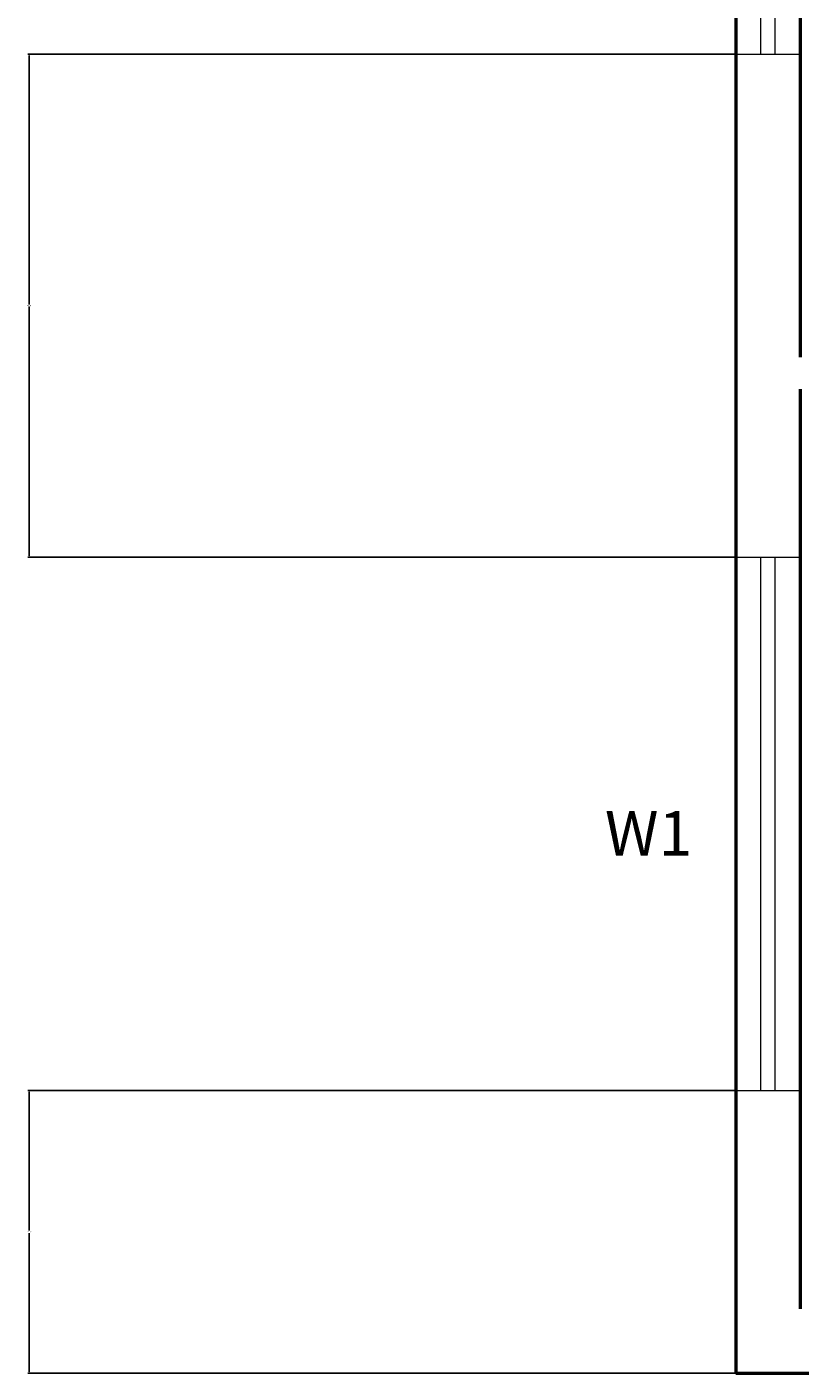
# Model space of a CAD drawing. Units: inches. Extents: x 7359 to 7979, y 33027 to 34263.
# Tile 2 of 32: x 7369 to 7478, y 33159 to 33347. Entities that reach past the tile are written whole.
import ezdxf

# ---------------------------------------------------------------- set-up
doc = ezdxf.new("R2010")
doc.units = ezdxf.units.IN
for name, color, linetype, lineweight in [('A-ANNO-DIMS', 2, 'Continuous', 18), ('A-ANNO-TEXT', 3, 'Continuous', 18), ('A-GLAZ', 4, 'Continuous', 18), ('A-WALL', 7, 'Continuous', 50)]:
    doc.layers.add(name, color=color, linetype=linetype, lineweight=lineweight)
doc.styles.get("Standard").update_dxf_attribs({"font": 'arial.ttf'})
doc.dimstyles.get("Standard").update_dxf_attribs({"dimtxt": 0.18, "dimasz": 0.18, "dimexe": 0.18, "dimexo": 0.0625, "dimgap": 0.09, "dimtad": 0, "dimtih": 1, "dimtoh": 1, "dimdec": 4, "dimzin": 0, "dimdsep": 46, "dimtxsty": 'Standard', "dimcen": 0.09, "dimadec": 0, "dimazin": 0, "dimtfac": 1, "dimtdec": 4, "dimtofl": 0, "dimtmove": 0, "dimatfit": 3, "dimfxl": 1, "dimtolj": 1, "dimtzin": 0, "dimarcsym": 0})

# ---------------------------------------------------------------- blocks, each defined once
blk = doc.blocks.new('WINDOW-W1-LIVING')
for p, q in [((0, 91.75), (9, 91.75)), ((3.5, 0), (3.5, 91.75)), ((5.5, 0), (5.5, 91.75)), ((0, 0), (9, 0))]:
    blk.add_line(p, q)
blk = doc.blocks.new('WINDOW-W1-DRAWING-SIDE')
for p, q in [((0, 74.75), (9, 74.75)), ((3.5, 0), (3.5, 74.75)), ((5.5, 0), (5.5, 74.75)), ((0, 0), (9, 0))]:
    blk.add_line(p, q)
blk = doc.blocks.new('*D79')
at = {"layer": 'A-ANNO-DIMS', "color": 0, "lineweight": -2, "transparency": 16777216}
for p, q in [((7468.66, 33198.25), (7369.54, 33198.25)), ((7369.72, 33198.07), (7369.72, 33178.64)), ((7369.72, 33158.84), (7369.72, 33178.28)), ((7468.66, 33158.66), (7369.54, 33158.66))]:
    blk.add_line(p, q, dxfattribs=at)
at = {"layer": 'A-ANNO-DIMS', "color": 0, "transparency": 16777216}
for points in [[(7369.69, 33198.07), (7369.75, 33198.07), (7369.72, 33198.25)], [(7369.69, 33158.84), (7369.75, 33158.84), (7369.72, 33158.66)]]:
    blk.add_solid(points, dxfattribs=at)
at = {"layer": 'Defpoints', "color": 0, "transparency": 16777216}
for p in [(7369.72, 33198.25), (7468.73, 33198.25), (7468.73, 33158.66)]:
    blk.add_point(p, dxfattribs=at)
at = {"layer": 'A-ANNO-DIMS', "color": 0, "transparency": 16777216, "insert": (7369.72, 33178.46), "char_height": 0.18, "attachment_point": 5}
blk.add_mtext('\\A1;39.59', dxfattribs=at)
blk = doc.blocks.new('*D80')
at = {"layer": 'A-ANNO-DIMS', "color": 0, "lineweight": -2, "transparency": 16777216}
for p, q in [((7468.66, 33343.52), (7369.54, 33343.52)), ((7369.72, 33343.34), (7369.72, 33308.44)), ((7369.72, 33273.18), (7369.72, 33308.08)), ((7468.66, 33273), (7369.54, 33273))]:
    blk.add_line(p, q, dxfattribs=at)
at = {"layer": 'A-ANNO-DIMS', "color": 0, "transparency": 16777216}
for points in [[(7369.69, 33343.34), (7369.75, 33343.34), (7369.72, 33343.52)], [(7369.69, 33273.18), (7369.75, 33273.18), (7369.72, 33273)]]:
    blk.add_solid(points, dxfattribs=at)
at = {"layer": 'Defpoints', "color": 0, "transparency": 16777216}
for p in [(7369.72, 33343.52), (7468.73, 33343.52), (7468.73, 33273)]:
    blk.add_point(p, dxfattribs=at)
at = {"layer": 'A-ANNO-DIMS', "color": 0, "transparency": 16777216, "insert": (7369.72, 33308.26), "char_height": 0.18, "attachment_point": 5}
blk.add_mtext('\\A1;70.51', dxfattribs=at)

msp = doc.modelspace()

# ---------------------------------------------------------------- linework, layer by layer
at = {"layer": 'A-WALL'}
for p, q in [((7468.7266, 33627.1623), (7468.7266, 33158.6623)), ((7477.7266, 33471.1623), (7477.7266, 33301.0623)), ((7477.7266, 33296.5623), (7477.7266, 33167.6623)), ((7468.7266, 33158.6623), (7894.1266, 33158.6623))]:
    msp.add_line(p, q, dxfattribs=at)

# ---------------------------------------------------------------- block references
at = {"layer": 'A-GLAZ'}
for name, p in [('WINDOW-W1-LIVING', (7468.7261, 33343.5154)), ('WINDOW-W1-DRAWING-SIDE', (7468.7261, 33198.2534))]:
    msp.add_blockref(name, p, dxfattribs=at)

# ---------------------------------------------------------------- texts
at = {"layer": 'A-ANNO-TEXT'}
msp.add_text('W1', height=6.25941, dxfattribs=at).set_placement((7450.3922, 33231.1644))

# ---------------------------------------------------------------- dimensions: what is measured, and where the dimension line sits
at = {"layer": 'A-ANNO-DIMS'}
for base, p1, p2, picture, middle in [((7369.7217, 33343.5157), (7468.7266, 33273.0048), (7468.7266, 33343.5157), '*D80', (7369.7217, 33308.2602)), ((7369.7217, 33198.2537), (7468.7266, 33158.6623), (7468.7266, 33198.2537), '*D79', (7369.7217, 33178.458))]:
    dim = msp.add_linear_dim(base=base, p1=p1, p2=p2, angle=90, dimstyle='Standard', override={"dimdec": 2, "dimlfac": 1, "dimrnd": 0, "dimzin": 0, "dimdsep": 46, "dimlunit": 2}, dxfattribs=at)
    dim.commit()
    dim.dimension.update_dxf_attribs({"geometry": picture, "text_midpoint": middle})

doc.saveas('drawing.dxf')
